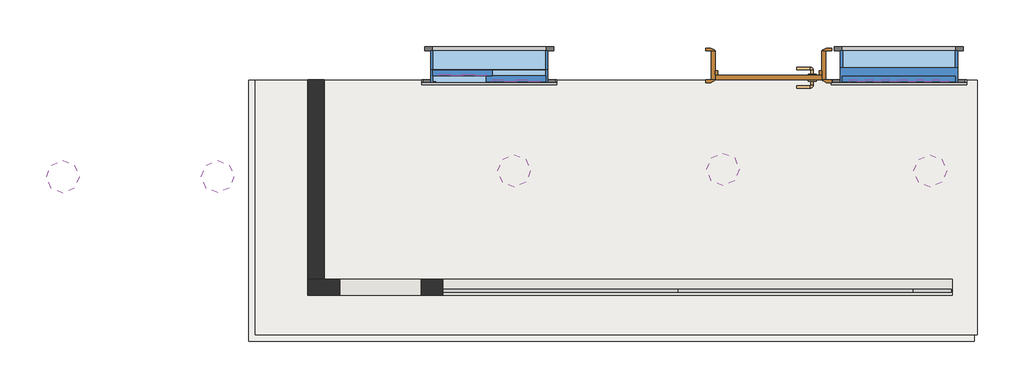
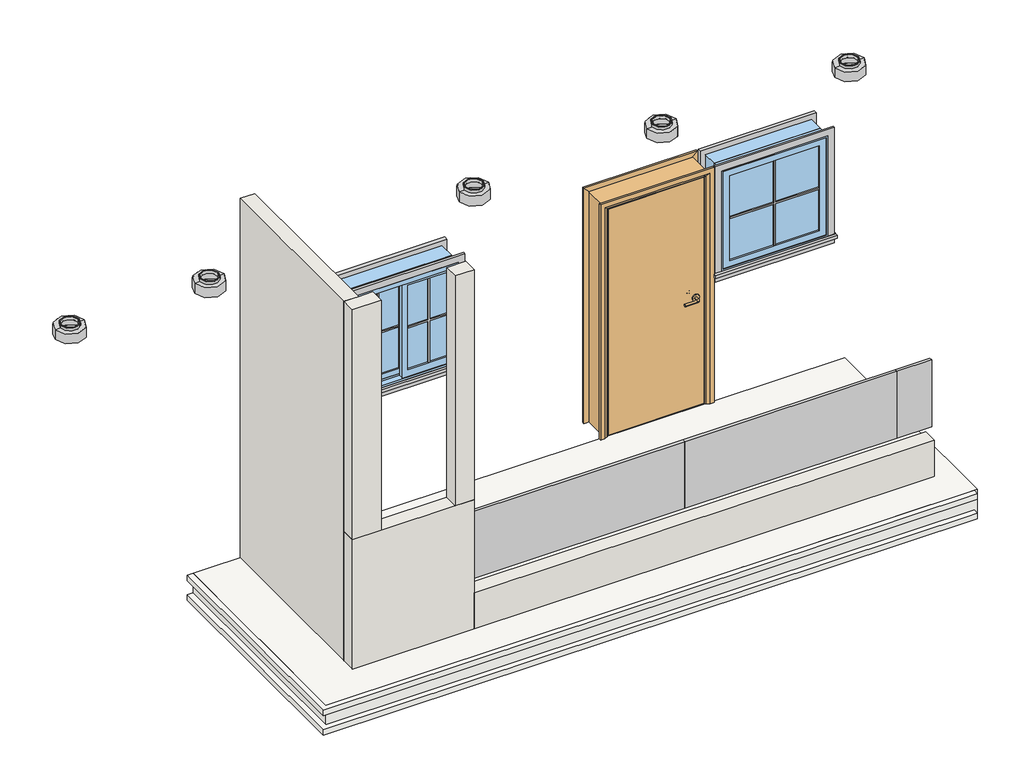
# One storey, incomplete: 7 proxies, 5 light fixtures, 5 walls, 3 plates, 3 slabs, 2 windows, 1 door.
"""IFC4 building model written with IfcOpenShell, lengths in millimetres."""

from ifc_helpers import new_model, si_unit, frame, origin, place, context, project, spatial, polyline, outline, extrude, faceted_brep, transform, mapped, element, save
from components import muntin_pattern_2x2_muntin_pattern_2x2_5e7f5336, muntin_pattern_2x2_muntin_pattern_2x2_37eac659, trim_window_exterior_flat_with_sill_84e24481, trim_window_interior_flat_picture_frame_28d4e5dc, doors_intsgl_910x2110mm_6866c2a0, ceiling_light_flat_round_60w_120v_7c4c2a52, system_panel_glazed_2daceabd, system_panel_glazed_face1e6f, window_df0b8b67, window_3ee5ce78

model = new_model("IFC4")

# Units and contexts
model_context = context("Model", 3, world=origin())
ifc_project = project(units=[si_unit("LENGTHUNIT", "METRE", prefix="MILLI")], contexts=[model_context])

# Site, building, storey
site = spatial("IfcSite", under=ifc_project)
building = spatial("IfcBuilding", under=site)
storey = spatial("IfcBuildingStorey", under=building, Elevation=8382.0)

# Proxies
placement = place(None, origin())
muntin_pattern_2x2_muntin_pattern_2x2_shape = muntin_pattern_2x2_muntin_pattern_2x2_5e7f5336(model_context)
element("IfcBuildingElementProxy", 1, Name="Muntin Pattern_2x2 : Muntin Pattern_2x2", ObjectType="Muntin Pattern_2x2 : Muntin Pattern_2x2", at=placement, inside=storey, context=model_context, shape_type="MappedRepresentation", body=[
    mapped(muntin_pattern_2x2_muntin_pattern_2x2_shape, transform((4401.3097446, -6872.0303244, 9603.0668667), x_axis=(-1.0, 0.0, 0.0), y_axis=(0.0, -1.0, 0.0), z_axis=(0.0, 0.0, 1.0))),
])
element("IfcBuildingElementProxy", 2, Name="Muntin Pattern_2x2 : Muntin Pattern_2x2", ObjectType="Muntin Pattern_2x2 : Muntin Pattern_2x2", at=placement, inside=storey, context=model_context, shape_type="MappedRepresentation", body=[
    mapped(muntin_pattern_2x2_muntin_pattern_2x2_shape, transform((4817.2347446, -6916.4803244, 9603.0668667), x_axis=(-1.0, 0.0, 0.0), y_axis=(0.0, -1.0, 0.0), z_axis=(0.0, 0.0, 1.0))),
])
muntin_pattern_2x2_muntin_pattern_2x2_2_shape = muntin_pattern_2x2_muntin_pattern_2x2_37eac659(model_context)
element("IfcBuildingElementProxy", 3, Name="Muntin Pattern_2x2 : Muntin Pattern_2x2", ObjectType="Muntin Pattern_2x2 : Muntin Pattern_2x2", at=placement, inside=storey, context=model_context, shape_type="MappedRepresentation", body=[
    mapped(muntin_pattern_2x2_muntin_pattern_2x2_2_shape, transform((7797.1305046, -6916.4803244, 9625.1936332), x_axis=(-1.0, 0.0, 0.0), y_axis=(0.0, -1.0, 0.0), z_axis=(0.0, 0.0, 1.0))),
])
trim_window_exterior_flat_with_sill_shape = trim_window_exterior_flat_with_sill_84e24481(model_context)
element("IfcBuildingElementProxy", 4, Name="Trim-Window-Exterior-Flat : with Sill", ObjectType="Trim-Window-Exterior-Flat : with Sill", at=placement, inside=storey, context=model_context, shape_type="MappedRepresentation", body=[
    mapped(trim_window_exterior_flat_with_sill_shape, transform((7797.1305046, -6926.0053244, 10469.7436332), x_axis=(1.0, 0.0, 0.0), y_axis=(0.0, 0.0, 1.0), z_axis=(0.0, -1.0, 0.0))),
])
element("IfcBuildingElementProxy", 5, Name="Trim-Window-Exterior-Flat : with Sill", ObjectType="Trim-Window-Exterior-Flat : with Sill", at=placement, inside=storey, context=model_context, shape_type="MappedRepresentation", body=[
    mapped(trim_window_exterior_flat_with_sill_shape, transform((4609.2722446, -6926.0053244, 10434.9168667), x_axis=(1.0, 0.0, 0.0), y_axis=(0.0, 0.0, 1.0), z_axis=(0.0, -1.0, 0.0))),
])
trim_window_interior_flat_picture_frame_shape = trim_window_interior_flat_picture_frame_28d4e5dc(model_context)
element("IfcBuildingElementProxy", 6, Name="Trim-Window-Interior-Flat : Picture Frame", ObjectType="Trim-Window-Interior-Flat : Picture Frame", at=placement, inside=storey, context=model_context, shape_type="MappedRepresentation", body=[
    mapped(trim_window_interior_flat_picture_frame_shape, transform((7797.1305046, -6697.4053244, 10469.7436332), x_axis=(-1.0, 0.0, 0.0), y_axis=(0.0, 0.0, 1.0), z_axis=(0.0, 1.0, 0.0))),
])
element("IfcBuildingElementProxy", 7, Name="Trim-Window-Interior-Flat : Picture Frame", ObjectType="Trim-Window-Interior-Flat : Picture Frame", at=placement, inside=storey, context=model_context, shape_type="MappedRepresentation", body=[
    mapped(trim_window_interior_flat_picture_frame_shape, transform((4609.2722446, -6697.4053244, 10434.9168667), x_axis=(-1.0, 0.0, 0.0), y_axis=(0.0, 0.0, 1.0), z_axis=(0.0, 1.0, 0.0))),
])

# Door
doors_intsgl_910x2110mm_shape = doors_intsgl_910x2110mm_6866c2a0(model_context)
element("IfcDoor", 8, ObjectType="Doors_IntSgl : 910x2110mm", at=placement, inside=storey, context=model_context, shape_type="MappedRepresentation", body=[
    mapped(doors_intsgl_910x2110mm_shape, transform((6783.3305046, -6811.7053244, 8382.0), x_axis=(-1.0, 0.0, 0.0), y_axis=(0.0, -1.0, 0.0), z_axis=(0.0, 0.0, 1.0))),
])

# Light fixtures
ceiling_light_flat_round_60w_120v_shape = ceiling_light_flat_round_60w_120v_7c4c2a52(model_context)
element("IfcLightFixture", 9, ObjectType="Ceiling Light - Flat Round : 60W - 120V", at=placement, inside=storey, context=model_context, shape_type="MappedRepresentation", body=[
    mapped(ceiling_light_flat_round_60w_120v_shape, transform((1290.2503416, -7679.1163795, 9217.6203125), x_axis=(1.0, 0.0, 0.0), y_axis=(0.0, 1.0, 0.0), z_axis=(0.0, 0.0, 1.0))),
])
element("IfcLightFixture", 10, ObjectType="Ceiling Light - Flat Round : 60W - 120V", at=placement, inside=storey, context=model_context, shape_type="MappedRepresentation", body=[
    mapped(ceiling_light_flat_round_60w_120v_shape, transform((2494.8977326, -7678.0859617, 9217.6203125), x_axis=(1.0, 0.0, 0.0), y_axis=(0.0, 1.0, 0.0), z_axis=(0.0, 0.0, 1.0))),
])
element("IfcLightFixture", 11, ObjectType="Ceiling Light - Flat Round : 60W - 120V", at=placement, inside=storey, context=model_context, shape_type="MappedRepresentation", body=[
    mapped(ceiling_light_flat_round_60w_120v_shape, transform((4802.7897682, -7633.7845831, 9217.6203125), x_axis=(1.0, 0.0, 0.0), y_axis=(0.0, 1.0, 0.0), z_axis=(0.0, 0.0, 1.0))),
])
element("IfcLightFixture", 12, ObjectType="Ceiling Light - Flat Round : 60W - 120V", at=placement, inside=storey, context=model_context, shape_type="MappedRepresentation", body=[
    mapped(ceiling_light_flat_round_60w_120v_shape, transform((6428.3868005, -7621.7105729, 9217.6203125), x_axis=(1.0, 0.0, 0.0), y_axis=(0.0, 1.0, 0.0), z_axis=(0.0, 0.0, 1.0))),
])
element("IfcLightFixture", 13, ObjectType="Ceiling Light - Flat Round : 60W - 120V", at=placement, inside=storey, context=model_context, shape_type="MappedRepresentation", body=[
    mapped(ceiling_light_flat_round_60w_120v_shape, transform((8041.5360018, -7634.3112335, 9217.6203125), x_axis=(1.0, 0.0, 0.0), y_axis=(0.0, 1.0, 0.0), z_axis=(0.0, 0.0, 1.0))),
])

# Plates
system_panel_glazed_shape = system_panel_glazed_2daceabd(model_context)
element("IfcPlate", 14, ObjectType="System Panel : Glazed", at=placement, inside=storey, context=model_context, shape_type="MappedRepresentation", body=[
    mapped(system_panel_glazed_shape, transform((5160.9441179, -8602.4053244, 8825.3327887), x_axis=(1.0, 0.0, 0.0), y_axis=(0.0, 1.0, 0.0), z_axis=(0.0, 0.0, 1.0))),
])
element("IfcPlate", 15, ObjectType="System Panel : Glazed", at=placement, inside=storey, context=model_context, shape_type="MappedRepresentation", body=[
    mapped(system_panel_glazed_shape, transform((6990.944118, -8602.4053244, 8825.3327887), x_axis=(1.0, 0.0, 0.0), y_axis=(0.0, 1.0, 0.0), z_axis=(0.0, 0.0, 1.0))),
])
system_panel_glazed_2_shape = system_panel_glazed_face1e6f(model_context)
element("IfcPlate", 16, ObjectType="System Panel : Glazed", at=placement, inside=storey, context=model_context, shape_type="MappedRepresentation", body=[
    mapped(system_panel_glazed_2_shape, transform((8055.8353108, -8602.4053244, 8825.3327887), x_axis=(1.0, 0.0, 0.0), y_axis=(0.0, 1.0, 0.0), z_axis=(0.0, 0.0, 1.0))),
])

# Slabs
element("IfcSlab", 17, ObjectType="5\"", at=placement, inside=storey, context=model_context, shape_type="SweptSolid", body=[
    extrude(outline(polyline([(8382.7225473, -8907.2053244), (8382.7225473, -8958.0053244), (2738.5851432, -8958.0053244), (2738.5851432, -6926.0053244), (2789.467819, -6926.0053244), (2789.467819, -8907.2053244), (8382.7225473, -8907.2053244)])), frame((0.0, 0.0, 8331.2), z_axis=(0.0, 0.0, 1.0), x_axis=(1.0, 0.0, 0.0)), (0.0, 0.0, 1.0), 50.8),
])
element("IfcSlab", 18, ObjectType="5\"", at=placement, inside=storey, context=model_context, shape_type="SweptSolid", body=[
    extrude(outline(polyline([(8382.7225473, -8907.2053244), (8382.7225473, -8958.0053244), (2738.5851432, -8958.0053244), (2738.5851432, -6926.0053244), (2789.467819, -6926.0053244), (2789.467819, -8907.2053244), (8382.7225473, -8907.2053244)])), frame((0.0, 0.0, 8153.4), z_axis=(0.0, 0.0, 1.0), x_axis=(1.0, 0.0, 0.0)), (0.0, 0.0, 1.0), 50.8),
])
element("IfcSlab", 19, ObjectType="9\"", at=placement, inside=storey, context=model_context, shape_type="SweptSolid", body=[
    extrude(outline(polyline([(8409.3004948, -6926.0053244), (8409.3004948, -8907.2053244), (2789.467819, -8907.2053244), (2789.467819, -6926.0053244), (8409.3004948, -6926.0053244)])), frame((0.0, 0.0, 8153.4), z_axis=(0.0, 0.0, 1.0), x_axis=(1.0, 0.0, 0.0)), (0.0, 0.0, 1.0), 228.6),
])

# Walls
element("IfcWall", 20, ObjectType="5\"", at=placement, inside=storey, context=model_context, shape_type="Brep", body=[
    faceted_brep([(3195.9504948, -8602.4053244, 8382.0), (4245.9441177, -8602.4053244, 8382.0), (4245.9441177, -8602.4053244, 8712.2), (4245.9441177, -8602.4053244, 9561.9327887), (4080.8441177, -8602.4053244, 9561.9327887), (3443.6004948, -8602.4053244, 9561.9327887), (3195.9504948, -8602.4053244, 9561.9327887), (3195.9504948, -8475.4053244, 8382.0), (3195.9504948, -8475.4053244, 9561.9327887), (3443.6004948, -8475.4053244, 9561.9327887), (4080.8441177, -8475.4053244, 9561.9327887), (4245.9441177, -8475.4053244, 9561.9327887), (4245.9441177, -8475.4053244, 8712.2), (4245.9441177, -8475.4053244, 8382.0), (3322.9504948, -8475.4053244, 8382.0)], [[[0, 1, 2, 3, 4, 5, 6]], [[7, 8, 9, 10, 11, 12, 13, 14]], [[1, 0, 7, 14, 13]], [[3, 2, 1, 13, 12, 11]], [[6, 5, 4, 3, 11, 10, 9, 8]], [[0, 6, 8, 7]]]),
])
element("IfcWall", 21, ObjectType="5\"", at=placement, inside=storey, context=model_context, shape_type="Brep", body=[
    faceted_brep([(3322.9504948, -8475.4053244, 11658.6), (3322.9504948, -8475.4053244, 8382.0), (3322.9504948, -6926.0053244, 8382.0), (3322.9504948, -6926.0053244, 11658.6), (3195.9504948, -8475.4053244, 8382.0), (3195.9504948, -8475.4053244, 9561.9327887), (3195.9504948, -8475.4053244, 11658.6), (3195.9504948, -6926.0053244, 11658.6), (3195.9504948, -6926.0053244, 8382.0)], [[[0, 1, 2, 3]], [[4, 5, 6, 7, 8]], [[2, 1, 4, 8]], [[0, 3, 7, 6]], [[3, 2, 8, 7]], [[0, 6, 5, 4, 1]]]),
])
element("IfcWall", 22, ObjectType="5\"", at=placement, inside=storey, context=model_context, shape_type="SweptSolid", body=[
    extrude(outline(polyline([(8213.5096373, -8602.4053244), (4245.9441177, -8602.4053244), (4245.9441177, -8475.4053244), (8213.5096373, -8475.4053244), (8213.5096373, -8602.4053244)])), frame((0.0, 0.0, 8382.0), z_axis=(0.0, 0.0, 1.0), x_axis=(1.0, 0.0, 0.0)), (0.0, 0.0, 1.0), 330.2),
])
element("IfcWall", 23, ObjectType="5\"", at=placement, inside=storey, context=model_context, shape_type="Brep", body=[
    faceted_brep([(4245.9441177, -8475.4053244, 9561.9327887), (4080.8441177, -8475.4053244, 9561.9327887), (4080.8441177, -8475.4053244, 11500.8069379), (4080.8441177, -8475.4053244, 11658.6), (4245.9441177, -8475.4053244, 11658.6), (4245.9441177, -8602.4053244, 9561.9327887), (4245.9441177, -8602.4053244, 11658.6), (4080.8441177, -8602.4053244, 11658.6), (4080.8441177, -8602.4053244, 11500.8069379), (4080.8441177, -8602.4053244, 9561.9327887)], [[[0, 1, 2, 3, 4]], [[5, 6, 7, 8, 9]], [[1, 0, 5, 9]], [[3, 2, 1, 9, 8, 7]], [[4, 3, 7, 6]], [[0, 4, 6, 5]]]),
])
element("IfcWall", 24, ObjectType="5\"", at=placement, inside=storey, context=model_context, shape_type="Brep", body=[
    faceted_brep([(3443.6004948, -8475.4053244, 9561.9327887), (3195.9504948, -8475.4053244, 9561.9327887), (3195.9504948, -8475.4053244, 11658.6), (3322.9504948, -8475.4053244, 11658.6), (3443.6004948, -8475.4053244, 11658.6), (3443.6004948, -8475.4053244, 11500.8069379), (3443.6004948, -8602.4053244, 9561.9327887), (3443.6004948, -8602.4053244, 11500.8069379), (3443.6004948, -8602.4053244, 11658.6), (3195.9504948, -8602.4053244, 11658.6), (3195.9504948, -8602.4053244, 9561.9327887)], [[[0, 1, 2, 3, 4, 5]], [[6, 7, 8, 9, 10]], [[1, 0, 6, 10]], [[4, 3, 2, 9, 8]], [[0, 5, 4, 8, 7, 6]], [[1, 10, 9, 2]]]),
])

# Windows
window_shape = window_df0b8b67(model_context)
element("IfcWindow", 25, ObjectType="Window-Casement-Single_Right : 36\" x 36\"", at=placement, inside=storey, context=model_context, shape_type="MappedRepresentation", body=[
    mapped(window_shape, transform((7797.1305046, -6811.7053244, 8640.9436332), x_axis=(-1.0, 0.0, 0.0), y_axis=(0.0, -1.0, 0.0), z_axis=(0.0, 0.0, 1.0))),
])
window_2_shape = window_3ee5ce78(model_context)
element("IfcWindow", 26, ObjectType="Window-Sliding-Double : 36\" x 36\"", at=placement, inside=storey, context=model_context, shape_type="MappedRepresentation", body=[
    mapped(window_2_shape, transform((4609.2722446, -6815.5153244, 8606.1168667), x_axis=(-1.0, 0.0, 0.0), y_axis=(0.0, -1.0, 0.0), z_axis=(0.0, 0.0, 1.0))),
])

save(model, "model.ifc")

# Revit data of these elements
# Type "Muntin Pattern_2x2 : Muntin Pattern_2x2"
#   Width [instance default] = 4' - 0"
#   Thickness = 0' - 0 1/2"
#   Height [instance default] = 4' - 0"
#   Distance = 0' - 0 3/4"
#   Interior Material [instance default] = none
#   Exterior Material [instance default] = none
#   Default Elevation = 0
# Type "Trim-Window-Exterior-Flat : with Sill"
#   Trim Width = 0' - 2 1/4"
#   Trim Thickness_Picture Frame = 0' - 1 1/4"
#   Trim Thickness_with Sill = 0' - 0 3/4"
#   Sill Thickness = 0' - 1 1/4"
#   Opening Width [instance default] = 2' - 0"
#   Opening Height [instance default] = 3' - 0"
#   Default Elevation = 4' - 0"
#   Sill = yes
#   Picture Frame = no
#   Trim Material [instance default] = none
# Type "Trim-Window-Interior-Flat : Picture Frame"
#   Trim Thickness_Picture Frame = 0' - 1 1/4"
#   Trim Width = 0' - 2 1/4"
#   Trim Thickness_with Sill = 0' - 0 3/4"
#   Sill Thickness = 0' - 1 1/4"
#   Opening Width [instance default] = 2' - 0"
#   Opening Height [instance default] = 3' - 0"
#   Default Elevation = 4' - 0"
#   Sill = no
#   Picture Frame = yes
#   Trim Material [instance default] = none
# Type "Doors_IntSgl : 910x2110mm"
#   Construction Type Id = "MDOOR"
#   Type Mark = "41"
#   Type Comments = "Internal Single"
#   Operation = "SingleSwingRight"
#   Manufacturer = "Revit"
#   Keynote = "L20"
#   Description = "Internal Single Door"
#   Analytic Construction = "Metal"
#   UnderCut = 0' - 0.31496"
#   Tolerance = 0' - 0.07874"
#   Thickness = 0' - 1.49606"
#   Thermal Resistance (R) = 0.270117 (m²·K)/W
#   Structural Tolerance = 0' - 0.31496"
#   StopDepth = 0' - 1.25984"
#   Stop Thickness = 0' - 0.74803"
#   Rough Width = 2' - 11.82677"
#   Rough Height = 6' - 11.07087"
#   Height to Top Lock Rail = 3' - 3.37008"
#   Heat Transfer Coefficient (U) = 3.7021 W/(m²·K)
#   Handle Z Distance = 3' - 3.37008"
#   Handle X Distance = 0' - 2.95276"
#   Frame Thickness = 0' - 1.25984"
#   Door Panel Width = 2' - 8.51969"
#   Door Panel Thickness = 0' - 1.49606"
#   Door Panel Offset = 0' - 0"
#   Height = 6' - 11.07087"
#   Width = 2' - 11.82677"
#   Door Panel Height = 6' - 9.10236"
#   Architrave Setback = 0' - 0.19685"
#   Define Thermal Properties by = 1
#   Vis - Ironmongery = yes
#   Material Ironmongery = Door - Handle
#   Material Frame = Door - Frame/Mullion (1)
#   Material Door = Door - Panel
#   Material Architrave = Door - Architrave
#   Visual Light Transmittance = 0
#   Solar Heat Gain Coefficient = 0
#   Function = (empty or 0)
#   Wall Closure = (empty or 0)
# Type "Ceiling Light - Flat Round : 60W - 120V"
#   Lamp = "A-19"
#   Assembly Code = "D5020220"
#   Wattage = 60 W
#   built-in parameter 1150110 = 1 (stored number, unit not read)
#   built-in parameter 1114217 = 1 (stored number, unit not read)
#   built-in parameter 1150109 = 1 (stored number, unit not read)
#   built-in parameter 1150113 = 1 (stored number, unit not read)
#   built-in parameter 1150115 = 1 (stored number, unit not read)
#   built-in parameter 1150105 = 272.155 (stored number, unit not read)
#   Light Source Symbol Size = 2' - 0"
#   built-in parameter 1150112 = 1 (stored number, unit not read)
#   built-in parameter 1150114 = 1 (stored number, unit not read)
#   built-in parameter 1150107 = 2800 (stored number, unit not read)
#   built-in parameter 1150106 = 2.72155 (stored number, unit not read)
#   Emit from Circle Diameter = 0' - 10"
#   built-in parameter 1150104 = 1.32387 (stored number, unit not read)
#   Ballast Voltage = 120 V
#   built-in parameter 1114218 = 1 (stored number, unit not read)
#   built-in parameter 1150133 = 10 (stored number, unit not read)
#   Lumens = 855 lm
#   Apparent Load = 60 VA
#   built-in parameter 1150134 = 4
#   built-in parameter 1150137 = 1
#   Color Filter = 16777215
#   built-in parameter 1140040 [instance default] = 1
#   Ballast Number of Poles = 1
#   Light Box Material = Steel, Paint Finish, Dark Gray, Matte
#   Diffuser Material = Glass, White, High Luminance
#   Wattage Comments = ""
#   Emit Shape Visible in Rendering = no
#   Dimming Lamp Color Temperature Shift = (empty or 0)
#   Default Elevation = 0
# Type "System Panel : Glazed"
#   Keynote = "H11"
#   Construction Type Id = "GSP4R"
#   Analytic Construction = "1/8 in Pilkington single glazing"
#   Visual Light Transmittance = 0.9
#   Solar Heat Gain Coefficient = 0.86
#   Heat Transfer Coefficient (U) = 6.7069 W/(m²·K)
#   Define Thermal Properties by = 1
# Type "5\""
#   Keynote = "E60/130"
#   Function = 0
#   Layers, outside or top first: 0' - 2" "Concrete, Precast" (function 1)
# Type "9\""
#   Keynote = "E60/130"
#   Function = 0
#   Layers, outside or top first: 0' - 9" "Concrete, Precast" (function 1)
# Type "5\""
#   Keynote = "F10"
#   Layers, outside or top first: 0' - 5" "Concrete" (function 1)
# Type "Window-Casement-Single_Right : 36\" x 36\""
#   Type Mark = "50"
#   Fire Rating = "0.5h"
#   Assembly Code = "B2020100"
#   Analytic Construction = "Double glazing - domestic"
#   Window Inset [instance default] = 0' - 0"
#   Wall Thickness [instance default] = 0' - 6"
#   Visual Light Transmittance = 0.81
#   Thermal Resistance (R) = 0.319569 (m²·K)/W
#   Solar Heat Gain Coefficient = 0.76
#   Rough Width = 3' - 0 1/2"
#   Rough Height = 3' - 0 1/2"
#   Interior Wall Closure [instance default] = 0' - 2 1/4"
#   Height = 3' - 0"
#   Heat Transfer Coefficient (U) = 3.12929 W/(m²·K)
#   Frame Extension [instance default] = 0' - 0 1/4"
#   Exterior Wall Closure [instance default] = 0' - 1 1/4"
#   Extension Jamb [instance default] = 0' - 2 1/4"
#   Default Sill Height = 3' - 0"
#   Width = 3' - 0"
#   Muntin Visibility = yes
#   Interior Trim Visibility [instance default] = yes
#   Exterior Trim Visibility [instance default] = yes
#   Extension Jamb Visibility [instance default] = yes
#   Muntin Pattern = Muntin Pattern_2x2 : Muntin Pattern_2x2
#   Interior Trim Material = Wood - Stained
#   Interior Trim = Trim-Window-Interior-Flat : Picture Frame
#   Interior Frame Material = Wood - Stained
#   Glass Panel Material = Glass
#   Exterior Trim Material = Clad - White
#   Exterior Trim = Trim-Window-Exterior-Flat : with Sill
#   Exterior Frame Material = Clad - White
#   Wall Closure = (empty or 0)
# Type "Window-Sliding-Double : 36\" x 36\""
#   Type Mark = "51"
#   Fire Rating = "0.5h"
#   Assembly Code = "B2020100"
#   Analytic Construction = "Double glazing - domestic"
#   Window Inset [instance default] = 0' - 0"
#   Wall Thickness [instance default] = 0' - 6"
#   Visual Light Transmittance = 0.81
#   Thermal Resistance (R) = 0.319569 (m²·K)/W
#   Solar Heat Gain Coefficient = 0.76
#   Muntin Width = 1' - 2 5/8"
#   Muntin Height = 2' - 6 1/4"
#   Interior Wall Closure [instance default] = 0' - 2 3/4"
#   Heat Transfer Coefficient (U) = 3.12929 W/(m²·K)
#   Frame Extension [instance default] = 0' - 0 1/4"
#   Exterior Wall Closure [instance default] = 0' - 1 1/4"
#   Rough Width = 3' - 0 1/2"
#   Rough Height = 3' - 0 1/2"
#   Height = 3' - 0"
#   Extension Jamb [instance default] = 0' - 2 3/4"
#   Default Sill Height = 3' - 0"
#   Width = 3' - 0"
#   Interior Trim Visibility [instance default] = yes
#   Indicator Visibility [instance default] = yes
#   Exterior Trim Visibility [instance default] = yes
#   Muntin Visibility = yes
#   Extension Jamb Visibility [instance default] = yes
#   Muntin Pattern = Muntin Pattern_2x2 : Muntin Pattern_2x2
#   Interior Trim Material = Wood - Stained
#   Interior Trim = Trim-Window-Interior-Flat : Picture Frame
#   Interior Frame Material = Wood - Stained
#   Glass Panel Material = Glass
#   Exterior Trim Material = Clad - White
#   Exterior Trim = Trim-Window-Exterior-Flat : with Sill
#   Exterior Frame Material = Clad - White
#   Wall Closure = (empty or 0)
# Elements 1, 2 (IfcBuildingElementProxy, "Muntin Pattern_2x2 : Muntin Pattern_2x2")
#   Width = 1' - 2 5/8"
#   Height = 2' - 6 1/4"
#   Interior Material = Wood - Stained
#   Exterior Material = Clad - White
#   Phase Created = New Construction
#   Materials on its faces: "Clad - White", "Wood - Stained"
# Element 3 (IfcBuildingElementProxy, "Muntin Pattern_2x2 : Muntin Pattern_2x2")
#   Width = 2' - 6 1/2"
#   Height = 2' - 6 1/2"
#   Interior Material = Wood - Stained
#   Exterior Material = Clad - White
#   Phase Created = New Construction
#   Materials on its faces: "Clad - White", "Wood - Stained"
# Elements 4, 5 (IfcBuildingElementProxy, "Trim-Window-Exterior-Flat : with Sill")
#   Opening Width = 3' - 0"
#   Opening Height = 3' - 0"
#   Trim Material = Clad - White
#   Phase Created = New Construction
#   Materials on its faces: "Clad - White"
# Elements 6, 7 (IfcBuildingElementProxy, "Trim-Window-Interior-Flat : Picture Frame")
#   Opening Width = 3' - 0"
#   Opening Height = 3' - 0"
#   Trim Material = Wood - Stained
#   Phase Created = New Construction
#   Materials on its faces: "Wood - Stained"
# Element 8 (IfcDoor, "Doors_IntSgl : 910x2110mm")
#   Phase Created = New Construction
#   Materials on its faces: "Door - Architrave", "Door - Handle", "Door - Frame/Mullion (1)", "Door - Panel"
# Element 9 (IfcLightFixture, "Ceiling Light - Flat Round : 60W - 120V")
#   Mark = "7"
#   built-in parameter 1140040 = 1
#   Phase Created = New Construction
#   Materials on its faces: "Glass, White, High Luminance", "Steel, Paint Finish, Dark Gray, Matte"
# Element 10 (IfcLightFixture, "Ceiling Light - Flat Round : 60W - 120V")
#   Mark = "8"
#   built-in parameter 1140040 = 1
#   Phase Created = New Construction
#   Materials on its faces: "Glass, White, High Luminance", "Steel, Paint Finish, Dark Gray, Matte"
# Element 11 (IfcLightFixture, "Ceiling Light - Flat Round : 60W - 120V")
#   Mark = "9"
#   built-in parameter 1140040 = 1
#   Phase Created = New Construction
#   Materials on its faces: "Glass, White, High Luminance", "Steel, Paint Finish, Dark Gray, Matte"
# Element 12 (IfcLightFixture, "Ceiling Light - Flat Round : 60W - 120V")
#   Mark = "10"
#   built-in parameter 1140040 = 1
#   Phase Created = New Construction
#   Materials on its faces: "Glass, White, High Luminance", "Steel, Paint Finish, Dark Gray, Matte"
# Element 13 (IfcLightFixture, "Ceiling Light - Flat Round : 60W - 120V")
#   Mark = "11"
#   built-in parameter 1140040 = 1
#   Phase Created = New Construction
#   Materials on its faces: "Glass, White, High Luminance", "Steel, Paint Finish, Dark Gray, Matte"
# Elements 14, 15, 16 (IfcPlate, "System Panel : Glazed")
#   Phase Created = New Construction
#   Materials on its faces: "Glass"
# Element 17 (IfcSlab, "5\"")
#   Height Offset From Level = 0' - 0"
#   Phase Created = New Construction
#   Materials on its faces: "Concrete, Precast"
# Element 18 (IfcSlab, "5\"")
#   Height Offset From Level = -0' - 7"
#   Phase Created = New Construction
#   Materials on its faces: "Concrete, Precast"
# Element 19 (IfcSlab, "9\"")
#   Height Offset From Level = 0' - 0"
#   Phase Created = New Construction
#   Materials on its faces: "Concrete, Precast"
# Element 20 (IfcWall, "5\"")
#   Top Offset = -7' - 7.54595"
#   Base Offset = 0' - 0"
#   wall height = 3' - 10.45405"
#   Phase Created = New Construction
#   Top Constraint = ROOF LEV
#   Materials on its faces: "Concrete"
# Element 21 (IfcWall, "5\"")
#   Top Offset = -0' - 9"
#   Base Offset = 0' - 0"
#   wall height = 10' - 9"
#   Phase Created = New Construction
#   Top Constraint = ROOF LEV
#   Materials on its faces: "Concrete"
# Element 22 (IfcWall, "5\"")
#   Top Offset = -10' - 0.54595"
#   Base Offset = 0' - 0"
#   wall height = 1' - 5.45405"
#   Phase Created = New Construction
#   Top Constraint = ROOF LEV
#   Materials on its faces: "Concrete"
# Elements 23, 24 (IfcWall, "5\"")
#   built-in parameter 1001111 = 3' - 10.45405"
#   Top Offset = -0' - 9"
#   Base Offset = 3' - 10.45405"
#   wall height = 6' - 10.54595"
#   Phase Created = New Construction
#   Top Constraint = ROOF LEV
#   Materials on its faces: "Concrete"
# Element 25 (IfcWindow, "Window-Casement-Single_Right : 36\" x 36\"")
#   Mark = "1"
#   Window Inset = 0' - 0"
#   Interior Wall Closure = 0' - 2 1/4"
#   Frame Extension = 0' - 0 1/4"
#   Exterior Wall Closure = 0' - 1 1/4"
#   Interior Trim Visibility = yes
#   Exterior Trim Visibility = yes
#   Phase Created = New Construction
#   Materials on its faces: "Wood - Stained", "Glass", "Clad - White"
# Element 26 (IfcWindow, "Window-Sliding-Double : 36\" x 36\"")
#   Mark = "2"
#   Window Inset = 0' - 0"
#   Interior Wall Closure = 0' - 2 3/4"
#   Frame Extension = 0' - 0 1/4"
#   Exterior Wall Closure = 0' - 1 1/4"
#   Interior Trim Visibility = yes
#   Indicator Visibility = yes
#   Exterior Trim Visibility = yes
#   Phase Created = New Construction
#   Materials on its faces: "Wood - Stained", "Glass", "Clad - White"
# Materials
#   "Door - Handle": colour RGB 0 0 0, transparency 0, Keynote = "P21", Cost = 0
#   "Door - Frame/Mullion (1)": class "Wood", colour RGB 212 179 113, transparency 0, Keynote = "L20", Cost = 0
#   "Door - Panel": class "Wood", colour RGB 210 159 95, transparency 0, Keynote = "L20", Cost = 0
#   "Door - Architrave": class "Wood", colour RGB 154 90 5, transparency 0, Keynote = "P20", Cost = 0
#   "Steel, Paint Finish, Dark Gray, Matte": class "Metal", colour RGB 98 98 98, transparency 0, Description = "Steel, paint finish, dark gray, matte", Cost = 0
#   "Glass, White, High Luminance": class "Glass", colour RGB 249 250 249, transparency 0.8, Description = "physical material", Cost = 0
#   "Concrete, Precast": class "Concrete", colour RGB 192 192 192, transparency 0, Description = "Precast concrete", Cost = 0
#   "Concrete": class "Concrete", colour RGB 120 120 120, transparency 0, Description = "Portland Cement Concrete", Cost = 0
#   "Wood - Stained": class "Wood", colour RGB 227 170 128, transparency 0, Cost = 0
#   "Glass": class "Glass", colour RGB 0 128 192, transparency 0.9, Description = "Soda Lime Glass", Cost = 0
#   "Clad - White": class "Wood", colour RGB 242 242 238, transparency 0, Cost = 0
